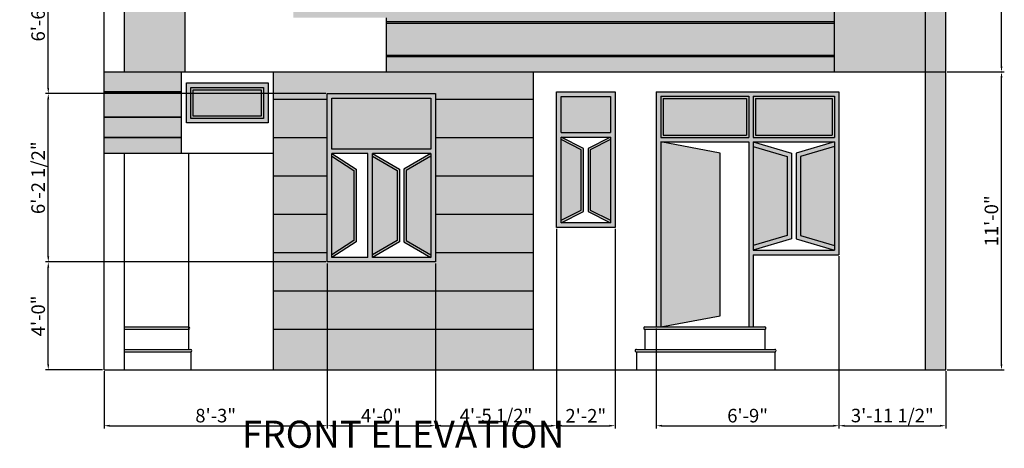
# Model space of a CAD drawing. Units: millimetres. Extents: x 4237 to 5109, y 21391 to 22486.
# Tile 1 of 17: x 4672 to 5109, y 21391 to 21581. Entities that reach past the tile are written whole.
import ezdxf

# ---------------------------------------------------------------- set-up
doc = ezdxf.new("R2010")
doc.units = ezdxf.units.MM
for name, color, linetype, lineweight in [('A-ANNO-DIMS', 2, 'Continuous', 18), ('A-ANNO-TEXT', 7, 'Continuous', 18), ('A-ELEV', 7, 'Continuous', 25), ('A-ELEV-PATT', 252, 'Continuous', 13)]:
    doc.layers.add(name, color=color, linetype=linetype, lineweight=lineweight)
doc.styles.get("Standard").update_dxf_attribs({"font": 'arial.ttf'})
doc.dimstyles.new('ISO-25', dxfattribs={"dimtxt": 6, "dimasz": 2.5, "dimexe": 1.25, "dimexo": 0.625, "dimtad": 1, "dimdec": 1, "dimlunit": 4, "dimtxsty": 'Standard', "dimcen": 2.5, "dimadec": 0, "dimazin": 0, "dimtfac": 1, "dimtdec": 1, "dimtmove": 0, "dimatfit": 3, "dimfxl": 1, "dimarcsym": 0})

# ---------------------------------------------------------------- blocks, each defined once
blk = doc.blocks.new('*D122')
at = {"layer": 'A-ANNO-DIMS', "color": 0, "lineweight": -2, "transparency": 16777216}
for p, q in [((4808.23, 21473.02), (4808.23, 21399.84)), ((4709.23, 21425.21), (4709.23, 21399.84)), ((4711.73, 21401.09), (4805.73, 21401.09))]:
    blk.add_line(p, q, dxfattribs=at)
at = {"layer": 'A-ANNO-DIMS', "color": 0, "transparency": 16777216}
for points in [[(4711.73, 21401.5), (4711.73, 21400.67), (4709.23, 21401.09)], [(4805.73, 21401.5), (4805.73, 21400.67), (4808.23, 21401.09)]]:
    blk.add_solid(points, dxfattribs=at)
at = {"layer": 'Defpoints', "color": 0, "transparency": 16777216}
for p in [(4808.23, 21473.65), (4709.23, 21425.84), (4808.23, 21401.09)]:
    blk.add_point(p, dxfattribs=at)
at = {"layer": 'A-ANNO-DIMS', "color": 0, "transparency": 16777216, "insert": (4758.73, 21404.78), "char_height": 6, "attachment_point": 5}
blk.add_mtext('8\'-3"', dxfattribs=at)
blk = doc.blocks.new('*D123')
at = {"layer": 'A-ANNO-DIMS', "color": 0, "lineweight": -2, "transparency": 16777216}
for p, q in [((4808.23, 21473.02), (4808.23, 21399.84)), ((4856.23, 21473.02), (4856.23, 21399.84)), ((4810.73, 21401.09), (4853.73, 21401.09))]:
    blk.add_line(p, q, dxfattribs=at)
at = {"layer": 'A-ANNO-DIMS', "color": 0, "transparency": 16777216}
for points in [[(4810.73, 21401.5), (4810.73, 21400.67), (4808.23, 21401.09)], [(4853.73, 21401.5), (4853.73, 21400.67), (4856.23, 21401.09)]]:
    blk.add_solid(points, dxfattribs=at)
at = {"layer": 'Defpoints', "color": 0, "transparency": 16777216}
for p in [(4808.23, 21473.65), (4856.23, 21473.65), (4856.23, 21401.09)]:
    blk.add_point(p, dxfattribs=at)
at = {"layer": 'A-ANNO-DIMS', "color": 0, "transparency": 16777216, "insert": (4832.23, 21404.77), "char_height": 6, "attachment_point": 5}
blk.add_mtext('4\'-0"', dxfattribs=at)
blk = doc.blocks.new('*D124')
at = {"layer": 'A-ANNO-DIMS', "color": 0, "lineweight": -2, "transparency": 16777216}
for p, q in [((4909.9, 21488.34), (4909.9, 21399.84)), ((4856.23, 21473.02), (4856.23, 21399.84)), ((4858.73, 21401.09), (4907.4, 21401.09))]:
    blk.add_line(p, q, dxfattribs=at)
at = {"layer": 'A-ANNO-DIMS', "color": 0, "transparency": 16777216}
for points in [[(4858.73, 21401.5), (4858.73, 21400.67), (4856.23, 21401.09)], [(4907.4, 21401.5), (4907.4, 21400.67), (4909.9, 21401.09)]]:
    blk.add_solid(points, dxfattribs=at)
at = {"layer": 'Defpoints', "color": 0, "transparency": 16777216}
for p in [(4909.9, 21488.97), (4856.23, 21473.65), (4909.9, 21401.09)]:
    blk.add_point(p, dxfattribs=at)
at = {"layer": 'A-ANNO-DIMS', "color": 0, "transparency": 16777216, "insert": (4883.06, 21404.81), "char_height": 6, "attachment_point": 5}
blk.add_mtext('4\'-5 1/2"', dxfattribs=at)
blk = doc.blocks.new('*D125')
at = {"layer": 'A-ANNO-DIMS', "color": 0, "lineweight": -2, "transparency": 16777216}
for p, q in [((4909.9, 21488.34), (4909.9, 21399.84)), ((4935.9, 21488.34), (4935.9, 21399.84)), ((4912.4, 21401.09), (4933.4, 21401.09))]:
    blk.add_line(p, q, dxfattribs=at)
at = {"layer": 'A-ANNO-DIMS', "color": 0, "transparency": 16777216}
for points in [[(4912.4, 21401.5), (4912.4, 21400.67), (4909.9, 21401.09)], [(4933.4, 21401.5), (4933.4, 21400.67), (4935.9, 21401.09)]]:
    blk.add_solid(points, dxfattribs=at)
at = {"layer": 'Defpoints', "color": 0, "transparency": 16777216}
for p in [(4909.9, 21488.97), (4935.9, 21488.97), (4935.9, 21401.09)]:
    blk.add_point(p, dxfattribs=at)
at = {"layer": 'A-ANNO-DIMS', "color": 0, "transparency": 16777216, "insert": (4922.9, 21404.72), "char_height": 6, "attachment_point": 5}
blk.add_mtext('2\'-2"', dxfattribs=at)
blk = doc.blocks.new('*D126')
at = {"layer": 'A-ANNO-DIMS', "color": 0, "lineweight": -2, "transparency": 16777216}
for p, q in [((5035.17, 21476.21), (5035.17, 21399.84)), ((4954.17, 21444.21), (4954.17, 21399.84)), ((4956.67, 21401.09), (5032.67, 21401.09))]:
    blk.add_line(p, q, dxfattribs=at)
at = {"layer": 'A-ANNO-DIMS', "color": 0, "transparency": 16777216}
for points in [[(4956.67, 21401.5), (4956.67, 21400.67), (4954.17, 21401.09)], [(5032.67, 21401.5), (5032.67, 21400.67), (5035.17, 21401.09)]]:
    blk.add_solid(points, dxfattribs=at)
at = {"layer": 'Defpoints', "color": 0, "transparency": 16777216}
for p in [(5035.17, 21476.84), (4954.17, 21444.84), (5035.17, 21401.09)]:
    blk.add_point(p, dxfattribs=at)
at = {"layer": 'A-ANNO-DIMS', "color": 0, "transparency": 16777216, "insert": (4994.67, 21404.77), "char_height": 6, "attachment_point": 5}
blk.add_mtext('6\'-9"', dxfattribs=at)
blk = doc.blocks.new('*D127')
at = {"layer": 'A-ANNO-DIMS', "color": 0, "lineweight": -2, "transparency": 16777216}
for p, q in [((5035.17, 21476.21), (5035.17, 21399.84)), ((5082.53, 21425.21), (5082.53, 21399.84)), ((5037.67, 21401.09), (5080.03, 21401.09))]:
    blk.add_line(p, q, dxfattribs=at)
at = {"layer": 'A-ANNO-DIMS', "color": 0, "transparency": 16777216}
for points in [[(5037.67, 21401.5), (5037.67, 21400.67), (5035.17, 21401.09)], [(5080.03, 21401.5), (5080.03, 21400.67), (5082.53, 21401.09)]]:
    blk.add_solid(points, dxfattribs=at)
at = {"layer": 'Defpoints', "color": 0, "transparency": 16777216}
for p in [(5035.17, 21476.84), (5082.53, 21425.84), (5082.53, 21401.09)]:
    blk.add_point(p, dxfattribs=at)
at = {"layer": 'A-ANNO-DIMS', "color": 0, "transparency": 16777216, "insert": (5058.85, 21404.82), "char_height": 6, "attachment_point": 5}
blk.add_mtext('3\'-11 1/2"', dxfattribs=at)
blk = doc.blocks.new('*D128')
at = {"layer": 'A-ANNO-DIMS', "color": 0, "lineweight": -2, "transparency": 16777216}
for p, q in [((4709.23, 21558.46), (4709.23, 21897.84)), ((4800.45, 21688.54), (4800.45, 21897.84)), ((4711.73, 21896.59), (4797.95, 21896.59))]:
    blk.add_line(p, q, dxfattribs=at)
at = {"layer": 'A-ANNO-DIMS', "color": 0, "transparency": 16777216}
for points in [[(4711.73, 21897), (4711.73, 21896.17), (4709.23, 21896.59)], [(4797.95, 21897), (4797.95, 21896.17), (4800.45, 21896.59)]]:
    blk.add_solid(points, dxfattribs=at)
at = {"layer": 'Defpoints', "color": 0, "transparency": 16777216}
for p in [(4800.45, 21896.59), (4800.45, 21687.91), (4709.23, 21557.84)]:
    blk.add_point(p, dxfattribs=at)
at = {"layer": 'A-ANNO-DIMS', "color": 0, "transparency": 16777216, "insert": (4754.84, 21900.21), "char_height": 6, "attachment_point": 5}
blk.add_mtext('7\'-7"', dxfattribs=at)
blk = doc.blocks.new('*D135')
at = {"layer": 'A-ANNO-DIMS', "color": 0, "lineweight": -2, "transparency": 16777216}
for p, q in [((5083.15, 21557.84), (5108.53, 21557.84)), ((5107.28, 21428.34), (5107.28, 21555.34)), ((5083.15, 21425.84), (5108.53, 21425.84))]:
    blk.add_line(p, q, dxfattribs=at)
at = {"layer": 'A-ANNO-DIMS', "color": 0, "transparency": 16777216}
for points in [[(5106.86, 21555.34), (5107.69, 21555.34), (5107.28, 21557.84)], [(5106.86, 21428.34), (5107.69, 21428.34), (5107.28, 21425.84)]]:
    blk.add_solid(points, dxfattribs=at)
at = {"layer": 'Defpoints', "color": 0, "transparency": 16777216}
for p in [(5082.53, 21557.84), (5107.28, 21557.84), (5082.53, 21425.84)]:
    blk.add_point(p, dxfattribs=at)
at = {"layer": 'A-ANNO-DIMS', "color": 0, "transparency": 16777216, "insert": (5103.59, 21491.84), "char_height": 6, "attachment_point": 5, "rotation": 90}
blk.add_mtext('11\'-0"', dxfattribs=at)
blk = doc.blocks.new('*D136')
at = {"layer": 'A-ANNO-DIMS', "color": 0, "lineweight": -2, "transparency": 16777216}
for p, q in [((5074.15, 21727.84), (5108.53, 21727.84)), ((5107.28, 21560.34), (5107.28, 21725.34)), ((5083.15, 21557.84), (5108.53, 21557.84))]:
    blk.add_line(p, q, dxfattribs=at)
at = {"layer": 'A-ANNO-DIMS', "color": 0, "transparency": 16777216}
for points in [[(5106.86, 21725.34), (5107.69, 21725.34), (5107.28, 21727.84)], [(5106.86, 21560.34), (5107.69, 21560.34), (5107.28, 21557.84)]]:
    blk.add_solid(points, dxfattribs=at)
at = {"layer": 'Defpoints', "color": 0, "transparency": 16777216}
for p in [(5073.53, 21727.84), (5107.28, 21727.84), (5082.53, 21557.84)]:
    blk.add_point(p, dxfattribs=at)
at = {"layer": 'A-ANNO-DIMS', "color": 0, "transparency": 16777216, "insert": (5103.64, 21642.84), "char_height": 6, "attachment_point": 5, "rotation": 90}
blk.add_mtext('14\'-2"', dxfattribs=at)
blk = doc.blocks.new('*D138')
at = {"layer": 'A-ANNO-DIMS', "color": 0, "lineweight": -2, "transparency": 16777216}
for p, q in [((4807.6, 21473.65), (4683.23, 21473.65)), ((4684.48, 21428.34), (4684.48, 21471.15)), ((4708.6, 21425.84), (4683.23, 21425.84))]:
    blk.add_line(p, q, dxfattribs=at)
at = {"layer": 'A-ANNO-DIMS', "color": 0, "transparency": 16777216}
for points in [[(4684.06, 21471.15), (4684.89, 21471.15), (4684.48, 21473.65)], [(4684.06, 21428.34), (4684.89, 21428.34), (4684.48, 21425.84)]]:
    blk.add_solid(points, dxfattribs=at)
at = {"layer": 'Defpoints', "color": 0, "transparency": 16777216}
for p in [(4684.48, 21473.65), (4808.23, 21473.65), (4709.23, 21425.84)]:
    blk.add_point(p, dxfattribs=at)
at = {"layer": 'A-ANNO-DIMS', "color": 0, "transparency": 16777216, "insert": (4680.79, 21449.74), "char_height": 6, "attachment_point": 5, "rotation": 90}
blk.add_mtext('4\'-0"', dxfattribs=at)
blk = doc.blocks.new('*D139')
at = {"layer": 'A-ANNO-DIMS', "color": 0, "lineweight": -2, "transparency": 16777216}
for p, q in [((4807.6, 21548.26), (4683.23, 21548.26)), ((4684.48, 21476.15), (4684.48, 21545.76)), ((4807.6, 21473.65), (4683.23, 21473.65))]:
    blk.add_line(p, q, dxfattribs=at)
at = {"layer": 'A-ANNO-DIMS', "color": 0, "transparency": 16777216}
for points in [[(4684.06, 21545.76), (4684.89, 21545.76), (4684.48, 21548.26)], [(4684.06, 21476.15), (4684.89, 21476.15), (4684.48, 21473.65)]]:
    blk.add_solid(points, dxfattribs=at)
at = {"layer": 'Defpoints', "color": 0, "transparency": 16777216}
for p in [(4684.48, 21548.26), (4808.23, 21548.26), (4808.23, 21473.65)]:
    blk.add_point(p, dxfattribs=at)
at = {"layer": 'A-ANNO-DIMS', "color": 0, "transparency": 16777216, "insert": (4680.75, 21510.96), "char_height": 6, "attachment_point": 5, "rotation": 90}
blk.add_mtext('6\'-2 1/2"', dxfattribs=at)
blk = doc.blocks.new('*D140')
at = {"layer": 'A-ANNO-DIMS', "color": 0, "lineweight": -2, "transparency": 16777216}
for p, q in [((4799.82, 21626.61), (4683.23, 21626.61)), ((4684.48, 21550.76), (4684.48, 21624.11)), ((4807.6, 21548.26), (4683.23, 21548.26))]:
    blk.add_line(p, q, dxfattribs=at)
at = {"layer": 'A-ANNO-DIMS', "color": 0, "transparency": 16777216}
for points in [[(4684.06, 21624.11), (4684.89, 21624.11), (4684.48, 21626.61)], [(4684.06, 21550.76), (4684.89, 21550.76), (4684.48, 21548.26)]]:
    blk.add_solid(points, dxfattribs=at)
at = {"layer": 'Defpoints', "color": 0, "transparency": 16777216}
for p in [(4684.48, 21626.61), (4800.45, 21626.61), (4808.23, 21548.26)]:
    blk.add_point(p, dxfattribs=at)
at = {"layer": 'A-ANNO-DIMS', "color": 0, "transparency": 16777216, "insert": (4680.75, 21587.44), "char_height": 6, "attachment_point": 5, "rotation": 90}
blk.add_mtext('6\'-6 1/2"', dxfattribs=at)

msp = doc.modelspace()

# ---------------------------------------------------------------- hatches: boundary and pattern name
at = {"layer": 'A-ELEV-PATT'}
h = msp.add_hatch(color=256, dxfattribs=at)
h.dxf.hatch_style = 1
h.paths.add_polyline_path([(4957.45, 21796.84), (4963.45, 21796.84), (4963.45, 21727.84), (4966.45, 21727.84), (4966.45, 21796.84), (4972.45, 21796.84), (4972.45, 21727.84), (4975.45, 21727.84), (4975.45, 21796.84), (4981.45, 21796.84), (4981.45, 21727.84), (4984.45, 21727.84), (4984.45, 21796.84), (5073.53, 21796.84), (5073.53, 21557.84), (5082.53, 21557.84), (5082.53, 21808.84), (4951.45, 21808.84), (4951.45, 21727.84), (4957.45, 21727.84)])
h = msp.add_hatch(color=256, dxfattribs=at)
h.dxf.hatch_style = 1
h.paths.add_polyline_path([(4763.12, 21763.84), (4718.23, 21763.84), (4718.23, 21557.84), (4745.15, 21557.84), (4745.15, 21725.84), (4742.84, 21725.84), (4742.84, 21727.84), (4763.12, 21727.84)])
h = msp.add_hatch(color=256, dxfattribs=at)
h.dxf.hatch_style = 1
h.paths.add_polyline_path([(5073.53, 21725.84), (5033.17, 21725.84), (5033.17, 21557.84), (5073.53, 21557.84)])
h = msp.add_hatch(color=256, dxfattribs=at)
h.dxf.hatch_style = 1
h.paths.add_polyline_path([(5033.17, 21587.38), (4793.12, 21587.38), (4793.12, 21581.84), (4834.56, 21581.84), (4834.56, 21580.12), (5033.17, 21580.12)])
h = msp.add_hatch(color=256, dxfattribs=at)
h.dxf.hatch_style = 1
h.paths.add_polyline_path([(5033.17, 21580.12), (4834.56, 21580.12), (4834.56, 21579.49), (5033.17, 21579.49)])
h = msp.add_hatch(color=256, dxfattribs=at)
h.dxf.hatch_style = 1
h.paths.add_polyline_path([(5033.17, 21579.49), (4834.56, 21579.49), (4834.56, 21565.26), (5033.17, 21565.26)])
h = msp.add_hatch(color=256, dxfattribs=at)
h.dxf.hatch_style = 1
h.paths.add_polyline_path([(5033.17, 21565.26), (4834.56, 21565.26), (4834.56, 21564.63), (5033.17, 21564.63)])
h = msp.add_hatch(color=256, dxfattribs=at)
h.dxf.hatch_style = 1
h.paths.add_polyline_path([(5033.17, 21564.63), (4834.56, 21564.63), (4834.56, 21557.84), (5033.17, 21557.84)])
h = msp.add_hatch(color=256, dxfattribs=at)
h.dxf.hatch_style = 1
h.paths.add_polyline_path([(4743.58, 21557.84), (4709.23, 21557.84), (4709.23, 21521.84), (4743.58, 21521.84)])
h = msp.add_hatch(color=256, dxfattribs=at)
h.dxf.hatch_style = 1
h.paths.add_polyline_path([(4899.53, 21557.84), (4784.23, 21557.84), (4784.23, 21425.84), (4899.53, 21425.84)])
h.paths.add_polyline_path([(4808.23, 21473.65), (4808.23, 21548.26), (4856.23, 21548.26), (4856.23, 21473.65)], flags=16)
h.paths.add_polyline_path([(4810.23, 21475.65), (4810.23, 21521.65), (4826.23, 21521.65), (4826.23, 21475.65)], flags=0)
h.paths.add_polyline_path([(4828.23, 21475.65), (4828.23, 21521.65), (4854.23, 21521.65), (4854.23, 21475.65)], flags=0)
h.paths.add_polyline_path([(4810.23, 21523.65), (4810.23, 21546.26), (4854.23, 21546.26), (4854.23, 21523.65)], flags=0)
h = msp.add_hatch(color=256, dxfattribs=at)
h.dxf.hatch_style = 1
h.paths.add_polyline_path([(5082.53, 21557.84), (5073.53, 21557.84), (5073.53, 21425.84), (5082.53, 21425.84)])
h = msp.add_hatch(color=256, dxfattribs=at)
h.dxf.hatch_style = 1
h.paths.add_polyline_path([(4781.97, 21552.96), (4745.76, 21552.96), (4745.76, 21535.28), (4781.97, 21535.28)])
h.paths.add_polyline_path([(4747.76, 21537.28), (4747.76, 21550.96), (4779.97, 21550.96), (4779.97, 21537.28)], flags=16)
h.paths.add_polyline_path([(4748.76, 21538.28), (4748.76, 21549.96), (4778.97, 21549.96), (4778.97, 21538.28)], flags=0)
h = msp.add_hatch(color=256, dxfattribs=at)
h.dxf.hatch_style = 1
h.set_gradient(color1=(122, 175, 223), color2=(215, 235, 210), name='CYLINDER')
h.paths.add_polyline_path([(4779.97, 21550.96), (4747.76, 21550.96), (4747.76, 21537.28), (4779.97, 21537.28)])
h.paths.add_polyline_path([(4778.97, 21538.28), (4748.76, 21538.28), (4748.76, 21549.96), (4778.97, 21549.96)], flags=16)
h = msp.add_hatch(color=256, dxfattribs=at)
h.dxf.hatch_style = 1
h.set_gradient(color1=(122, 175, 223), color2=(215, 235, 210), name='HEMISPHERICAL')
h.paths.add_polyline_path([(4778.97, 21549.96), (4748.76, 21549.96), (4748.76, 21538.28), (4778.97, 21538.28)])
h = msp.add_hatch(color=256, dxfattribs=at)
h.dxf.hatch_style = 1
h.paths.add_polyline_path([(4856.23, 21548.26), (4808.23, 21548.26), (4808.23, 21473.65), (4856.23, 21473.65)])
h.paths.add_polyline_path([(4854.23, 21546.26), (4854.23, 21523.65), (4810.23, 21523.65), (4810.23, 21546.26)], flags=16)
h.paths.add_polyline_path([(4854.23, 21521.65), (4854.23, 21475.65), (4828.23, 21475.65), (4828.23, 21521.65)], flags=16)
h.paths.add_polyline_path([(4826.23, 21521.65), (4826.23, 21475.65), (4810.23, 21475.65), (4810.23, 21521.65)], flags=16)
h = msp.add_hatch(color=256, dxfattribs=at)
h.dxf.hatch_style = 1
h.paths.add_polyline_path([(4935.9, 21548.97), (4909.9, 21548.97), (4909.9, 21488.97), (4935.9, 21488.97)])
h.paths.add_polyline_path([(4933.9, 21546.97), (4933.9, 21530.97), (4911.9, 21530.97), (4911.9, 21546.97)], flags=16)
h.paths.add_polyline_path([(4933.9, 21528.97), (4933.9, 21490.97), (4911.9, 21490.97), (4911.9, 21528.97)], flags=16)
h = msp.add_hatch(color=256, dxfattribs=at)
h.dxf.hatch_style = 1
h.paths.add_polyline_path([(5035.17, 21549.03), (4954.17, 21549.03), (4954.17, 21444.84), (4956.17, 21444.84), (4956.17, 21526.84), (4995.17, 21526.84), (4995.17, 21444.84), (4997.17, 21444.84), (4997.17, 21476.84), (5035.17, 21476.84)])
h.paths.add_polyline_path([(4995.17, 21547.03), (4995.17, 21528.84), (4956.17, 21528.84), (4956.17, 21547.03)], flags=16)
h.paths.add_polyline_path([(4994.17, 21546.03), (4994.17, 21529.84), (4957.17, 21529.84), (4957.17, 21546.03)], flags=0)
h.paths.add_polyline_path([(4997.17, 21547.03), (5033.17, 21547.03), (5033.17, 21528.84), (4997.17, 21528.84)], flags=16)
h.paths.add_polyline_path([(4998.17, 21546.03), (5032.17, 21546.03), (5032.17, 21529.84), (4998.17, 21529.84)], flags=0)
h.paths.add_polyline_path([(4997.17, 21526.84), (5033.17, 21526.84), (5033.17, 21478.84), (4997.17, 21478.84)], flags=16)
h = msp.add_hatch(color=256, dxfattribs=at)
h.dxf.hatch_style = 1
h.set_gradient(color1=(122, 175, 223), color2=(215, 235, 210), name='HEMISPHERICAL')
h.paths.add_polyline_path([(4854.23, 21546.26), (4810.23, 21546.26), (4810.23, 21523.65), (4854.23, 21523.65)])
h = msp.add_hatch(color=256, dxfattribs=at)
h.dxf.hatch_style = 1
h.set_gradient(color1=(122, 175, 223), color2=(215, 235, 210), name='HEMISPHERICAL')
h.paths.add_polyline_path([(4933.9, 21546.97), (4911.9, 21546.97), (4911.9, 21530.97), (4933.9, 21530.97)])
h = msp.add_hatch(color=256, dxfattribs=at)
h.dxf.hatch_style = 1
h.set_gradient(color1=(122, 175, 223), color2=(215, 235, 210), name='CYLINDER')
h.paths.add_polyline_path([(4995.17, 21547.03), (4956.17, 21547.03), (4956.17, 21528.84), (4995.17, 21528.84)])
h.paths.add_polyline_path([(4994.17, 21529.84), (4957.17, 21529.84), (4957.17, 21546.03), (4994.17, 21546.03)], flags=16)
h = msp.add_hatch(color=256, dxfattribs=at)
h.dxf.hatch_style = 1
h.set_gradient(color1=(122, 175, 223), color2=(215, 235, 210), name='HEMISPHERICAL')
h.paths.add_polyline_path([(4994.17, 21546.03), (4957.17, 21546.03), (4957.17, 21529.84), (4994.17, 21529.84)])
h = msp.add_hatch(color=256, dxfattribs=at)
h.dxf.hatch_style = 1
h.set_gradient(color1=(122, 175, 223), color2=(215, 235, 210), name='CYLINDER')
h.paths.add_polyline_path([(5033.17, 21547.03), (4997.17, 21547.03), (4997.17, 21528.84), (5033.17, 21528.84)])
h.paths.add_polyline_path([(4998.17, 21546.03), (5032.17, 21546.03), (5032.17, 21529.84), (4998.17, 21529.84)], flags=16)
h = msp.add_hatch(color=256, dxfattribs=at)
h.dxf.hatch_style = 1
h.set_gradient(color1=(122, 175, 223), color2=(215, 235, 210), name='HEMISPHERICAL')
h.paths.add_polyline_path([(5032.17, 21546.03), (4998.17, 21546.03), (4998.17, 21529.84), (5032.17, 21529.84)])
h = msp.add_hatch(color=256, dxfattribs=at)
h.dxf.hatch_style = 1
h.paths.add_polyline_path([(4921.9, 21523.97), (4911.9, 21528.97), (4911.9, 21527.85), (4920.9, 21523.35), (4920.9, 21496.59), (4911.9, 21492.09), (4911.9, 21490.97), (4921.9, 21495.97)])
h = msp.add_hatch(color=256, dxfattribs=at)
h.dxf.hatch_style = 1
h.set_gradient(color1=(122, 175, 223), color2=(215, 235, 210), name='INVCYLINDER')
h.paths.add_polyline_path([(4920.9, 21523.35), (4911.9, 21527.85), (4911.9, 21492.09), (4920.9, 21496.59)])
h = msp.add_hatch(color=256, dxfattribs=at)
h.dxf.hatch_style = 1
h.paths.add_polyline_path([(4924.9, 21523.35), (4933.9, 21527.85), (4933.9, 21528.97), (4923.9, 21523.97), (4923.9, 21495.97), (4933.9, 21490.97), (4933.9, 21492.09), (4924.9, 21496.59)])
h = msp.add_hatch(color=256, dxfattribs=at)
h.dxf.hatch_style = 1
h.set_gradient(color1=(122, 175, 223), color2=(215, 235, 210), name='INVCYLINDER')
h.paths.add_polyline_path([(4933.9, 21527.85), (4924.9, 21523.35), (4924.9, 21496.59), (4933.9, 21492.09)])
h = msp.add_hatch(color=256, dxfattribs=at)
h.dxf.hatch_style = 1
h.paths.add_polyline_path([(4982.51, 21521.84), (4956.17, 21526.84), (4956.17, 21444.84), (4982.51, 21449.84)])
h = msp.add_hatch(color=256, dxfattribs=at)
h.dxf.hatch_style = 1
h.paths.add_polyline_path([(5014.17, 21521.84), (4997.17, 21526.84), (4997.17, 21524.75), (5012.17, 21520.34), (5012.17, 21485.33), (4997.17, 21480.92), (4997.17, 21478.84), (5014.17, 21483.84)])
h = msp.add_hatch(color=256, dxfattribs=at)
h.dxf.hatch_style = 1
h.paths.add_polyline_path([(5018.17, 21520.34), (5033.17, 21524.75), (5033.17, 21526.84), (5016.17, 21521.84), (5016.17, 21483.84), (5033.17, 21478.84), (5033.17, 21480.92), (5018.17, 21485.33)])
h = msp.add_hatch(color=256, dxfattribs=at)
h.dxf.hatch_style = 1
h.set_gradient(color1=(122, 175, 223), color2=(215, 235, 210), name='INVCYLINDER')
h.paths.add_polyline_path([(5012.17, 21520.34), (4997.17, 21524.75), (4997.17, 21480.92), (5012.17, 21485.33)])
h = msp.add_hatch(color=256, dxfattribs=at)
h.dxf.hatch_style = 1
h.set_gradient(color1=(122, 175, 223), color2=(215, 235, 210), name='INVCYLINDER')
h.paths.add_polyline_path([(5033.17, 21524.75), (5018.17, 21520.34), (5018.17, 21485.33), (5033.17, 21480.92)])
h = msp.add_hatch(color=256, dxfattribs=at)
h.dxf.hatch_style = 1
h.paths.add_polyline_path([(4821, 21514.73), (4810.23, 21521.65), (4810.23, 21520.46), (4820, 21514.19), (4820, 21483.11), (4810.23, 21476.84), (4810.23, 21475.65), (4821, 21482.56)])
h = msp.add_hatch(color=256, dxfattribs=at)
h.dxf.hatch_style = 1
h.set_gradient(color1=(122, 175, 223), color2=(215, 235, 210), name='INVCYLINDER')
h.paths.add_polyline_path([(4820, 21514.19), (4810.23, 21520.46), (4810.23, 21476.84), (4820, 21483.11)])
h = msp.add_hatch(color=256, dxfattribs=at)
h.dxf.hatch_style = 1
h.paths.add_polyline_path([(4840.21, 21514.73), (4828.23, 21521.65), (4828.23, 21520.49), (4839.21, 21514.16), (4839.21, 21483.14), (4828.23, 21476.8), (4828.23, 21475.65), (4840.21, 21482.56)])
h = msp.add_hatch(color=256, dxfattribs=at)
h.dxf.hatch_style = 1
h.set_gradient(color1=(122, 175, 223), color2=(215, 235, 210), name='INVCYLINDER')
h.paths.add_polyline_path([(4839.21, 21514.16), (4828.23, 21520.49), (4828.23, 21476.8), (4839.21, 21483.14)])
h = msp.add_hatch(color=256, dxfattribs=at)
h.dxf.hatch_style = 1
h.paths.add_polyline_path([(4843.24, 21514.16), (4854.23, 21520.49), (4854.23, 21521.65), (4842.24, 21514.73), (4842.24, 21482.56), (4854.23, 21475.65), (4854.23, 21476.8), (4843.24, 21483.14)])
h = msp.add_hatch(color=256, dxfattribs=at)
h.dxf.hatch_style = 1
h.set_gradient(color1=(122, 175, 223), color2=(215, 235, 210), name='INVCYLINDER')
h.paths.add_polyline_path([(4854.23, 21520.49), (4843.24, 21514.16), (4843.24, 21483.14), (4854.23, 21476.8)])

# ---------------------------------------------------------------- linework, layer by layer
at = {"layer": 'A-ELEV'}
for p, q in [((4709.23, 21425.84), (4709.23, 21871.84)), ((5082.53, 21425.84), (5082.53, 21808.84)), ((5073.53, 21425.84), (5073.53, 21796.84)), ((5033.17, 21557.84), (5033.17, 21772.84)), ((4718.23, 21557.84), (4718.23, 21763.84)), ((4745.15, 21557.84), (4745.15, 21725.84)), ((4834.56, 21557.84), (4834.56, 21581.84)), ((4834.56, 21580.12), (5033.17, 21580.12)), ((4834.56, 21579.49), (5033.17, 21579.49)), ((4834.56, 21565.26), (5033.17, 21565.26)), ((4834.56, 21564.63), (5033.17, 21564.63)), ((4709.23, 21557.84), (5082.53, 21557.84)), ((4743.58, 21521.84), (4743.58, 21557.84)), ((4784.23, 21557.84), (4784.23, 21425.84)), ((4899.53, 21557.84), (4899.53, 21425.84)), ((4709.23, 21549.12), (4743.58, 21549.12)), ((4709.23, 21548.93), (4743.58, 21548.93)), ((4808.23, 21548.26), (4856.23, 21548.26)), ((4808.23, 21473.65), (4808.23, 21548.26)), ((4856.23, 21548.26), (4856.23, 21473.65)), ((4909.9, 21548.97), (4935.9, 21548.97)), ((4909.9, 21488.97), (4909.9, 21548.97)), ((4935.9, 21548.97), (4935.9, 21488.97)), ((4954.17, 21549.03), (4954.17, 21444.84)), ((4954.17, 21549.03), (5035.17, 21549.03)), ((5035.17, 21549.03), (5035.17, 21476.84)), ((4784.23, 21545.84), (4808.23, 21545.84)), ((4856.23, 21545.84), (4899.53, 21545.84)), ((4911.9, 21546.97), (4933.9, 21546.97)), ((4911.9, 21530.97), (4911.9, 21546.97)), ((4933.9, 21546.97), (4933.9, 21530.97)), ((4956.17, 21547.03), (4956.17, 21528.84)), ((4956.17, 21547.03), (4995.17, 21547.03)), ((4957.17, 21546.03), (4957.17, 21529.84)), ((4957.17, 21546.03), (4994.17, 21546.03)), ((4994.17, 21546.03), (4994.17, 21529.84)), ((4995.17, 21547.03), (4995.17, 21528.84)), ((4997.17, 21547.03), (4997.17, 21528.84)), ((4997.17, 21547.03), (5033.17, 21547.03)), ((4998.17, 21546.03), (4998.17, 21529.84)), ((4998.17, 21546.03), (5032.17, 21546.03)), ((5032.17, 21546.03), (5032.17, 21529.84)), ((5033.17, 21547.03), (5033.17, 21528.84)), ((4709.23, 21537.93), (4743.58, 21537.93)), ((4709.23, 21537.73), (4743.58, 21537.73)), ((4911.9, 21530.97), (4933.9, 21530.97)), ((4709.23, 21529.01), (4743.58, 21529.01)), ((4709.23, 21528.81), (4743.58, 21528.81)), ((4784.23, 21528.84), (4808.23, 21528.84)), ((4856.23, 21528.84), (4899.53, 21528.84)), ((4911.9, 21528.97), (4933.9, 21528.97)), ((4911.9, 21490.97), (4911.9, 21528.97)), ((4933.9, 21528.97), (4933.9, 21490.97)), ((4956.17, 21528.84), (4995.17, 21528.84)), ((4956.17, 21526.84), (4995.17, 21526.84)), ((4956.17, 21526.84), (4956.17, 21444.84)), ((4957.17, 21529.84), (4994.17, 21529.84)), ((4995.17, 21526.84), (4995.17, 21444.84)), ((4997.17, 21528.84), (5033.17, 21528.84)), ((4997.17, 21526.84), (5033.17, 21526.84)), ((4997.17, 21526.84), (4997.17, 21478.84)), ((4998.17, 21529.84), (5032.17, 21529.84)), ((5033.17, 21526.84), (5033.17, 21478.84)), ((4709.23, 21521.84), (4784.23, 21521.84)), ((4718.23, 21425.84), (4718.23, 21521.84)), ((4746.73, 21521.84), (4746.73, 21434.84)), ((4826.23, 21521.65), (4810.23, 21521.65)), ((4810.23, 21475.65), (4810.23, 21521.65)), ((4826.23, 21475.65), (4826.23, 21521.65)), ((4854.23, 21521.65), (4828.23, 21521.65)), ((4828.23, 21475.65), (4828.23, 21521.65)), ((4854.23, 21521.65), (4854.23, 21475.65)), ((4784.23, 21511.84), (4808.23, 21511.84)), ((4856.23, 21511.84), (4899.53, 21511.84)), ((4784.23, 21494.84), (4808.23, 21494.84)), ((4856.23, 21494.84), (4899.53, 21494.84)), ((4935.9, 21488.97), (4909.9, 21488.97)), ((4933.9, 21490.97), (4911.9, 21490.97)), ((4997.17, 21478.84), (5033.17, 21478.84)), ((4784.23, 21477.84), (4808.23, 21477.84)), ((4826.23, 21475.65), (4810.23, 21475.65)), ((4854.23, 21475.65), (4828.23, 21475.65)), ((4856.23, 21477.84), (4899.53, 21477.84)), ((4997.17, 21476.84), (5035.17, 21476.84)), ((4997.17, 21476.84), (4997.17, 21444.84)), ((4856.23, 21473.65), (4808.23, 21473.65)), ((4784.23, 21460.84), (4899.53, 21460.84)), ((4718.23, 21444.84), (4746.73, 21444.84)), ((4718.23, 21443.84), (4746.73, 21443.84)), ((4784.23, 21443.84), (4899.53, 21443.84)), ((4949.12, 21444.84), (5002.27, 21444.84)), ((4949.12, 21443.84), (5002.27, 21443.84)), ((4949.12, 21443.84), (4949.12, 21434.84)), ((5002.27, 21443.84), (5002.27, 21434.84)), ((4718.23, 21434.84), (4747.69, 21434.84)), ((4945.37, 21434.84), (5006.68, 21434.84)), ((4718.23, 21433.84), (4747.69, 21433.84)), ((4747.69, 21433.84), (4747.69, 21425.84)), ((4945.37, 21433.84), (5006.68, 21433.84)), ((4945.37, 21433.84), (4945.37, 21425.84)), ((5006.68, 21433.84), (5006.68, 21425.84)), ((4709.23, 21425.84), (5082.53, 21425.84))]:
    msp.add_line(p, q, dxfattribs=at)
for points in [[(4745.76, 21552.96), (4781.97, 21552.96), (4781.97, 21535.28), (4745.76, 21535.28)], [(4747.76, 21550.96), (4779.97, 21550.96), (4779.97, 21537.28), (4747.76, 21537.28)], [(4748.76, 21549.96), (4778.97, 21549.96), (4778.97, 21538.28), (4748.76, 21538.28)], [(4810.23, 21546.26), (4854.23, 21546.26), (4854.23, 21523.65), (4810.23, 21523.65)]]:
    msp.add_lwpolyline(points, close=True, dxfattribs=at)
for points in [[(4911.9, 21490.97), (4921.9, 21495.97), (4921.9, 21523.97), (4911.9, 21528.97)], [(4911.9, 21492.09), (4920.9, 21496.59), (4920.9, 21523.35), (4911.9, 21527.85)], [(4933.9, 21528.97), (4923.9, 21523.97), (4923.9, 21495.97), (4933.9, 21490.97)], [(4933.9, 21527.85), (4924.9, 21523.35), (4924.9, 21496.59), (4933.9, 21492.09)], [(4956.17, 21444.84), (4982.51, 21449.84), (4982.51, 21521.84), (4956.17, 21526.84)], [(4997.17, 21526.84), (5014.17, 21521.84), (5014.17, 21483.84), (4997.17, 21478.84)], [(5033.17, 21526.84), (5016.17, 21521.84), (5016.17, 21483.84), (5033.17, 21478.84)], [(4997.17, 21524.75), (5012.17, 21520.34), (5012.17, 21485.33), (4997.17, 21480.92)], [(5033.17, 21524.75), (5018.17, 21520.34), (5018.17, 21485.33), (5033.17, 21480.92)], [(4810.23, 21521.65), (4821, 21514.73), (4821, 21482.56), (4810.23, 21475.65)], [(4810.23, 21520.46), (4820, 21514.19), (4820, 21483.11), (4810.23, 21476.84)], [(4828.23, 21521.65), (4840.21, 21514.73), (4840.21, 21482.56), (4828.23, 21475.65)], [(4828.23, 21520.49), (4839.21, 21514.16), (4839.21, 21483.14), (4828.23, 21476.8)], [(4854.23, 21521.65), (4842.24, 21514.73), (4842.24, 21482.56), (4854.23, 21475.65)], [(4854.23, 21520.49), (4843.24, 21514.16), (4843.24, 21483.14), (4854.23, 21476.8)]]:
    msp.add_lwpolyline(points, dxfattribs=at)
for centre, radius, start, end in [((4746.74, 21444.34), 0.5, 268.0101, 91.9899), ((4949.08, 21444.34), 0.502, 84.9128, 275.0872), ((5002.31, 21444.34), 0.502, 264.751, 95.249), ((4747.69, 21434.34), 0.5, 270.7076, 89.2924), ((4945.24, 21434.34), 0.517, 75.0765, 284.9235), ((5006.77, 21434.34), 0.51, 258.8891, 101.1109)]:
    msp.add_arc(centre, radius, start, end, dxfattribs=at)

# ---------------------------------------------------------------- texts
at = {"layer": 'A-ANNO-TEXT', "insert": (4755.67, 21403.3), "char_height": 12, "attachment_point": 1}
msp.add_mtext_dynamic_manual_height_columns('    FRONT ELEVATION', width=222.3103, gutter_width=12.5, heights=[0], dxfattribs=at)

# ---------------------------------------------------------------- dimensions: what is measured, and where the dimension line sits
at = {"layer": 'A-ANNO-DIMS'}
for base, p1, p2, picture, middle in [((4800.45, 21896.59), (4709.23, 21557.84), (4800.45, 21687.91), '*D128', (4754.84, 21900.21)), ((4909.9, 21401.09), (4856.23, 21473.65), (4909.9, 21488.97), '*D124', (4883.06, 21404.81)), ((4935.9, 21401.09), (4909.9, 21488.97), (4935.9, 21488.97), '*D125', (4922.9, 21404.72)), ((5035.17, 21401.09), (4954.17, 21444.84), (5035.17, 21476.84), '*D126', (4994.67, 21404.77)), ((5082.53, 21401.09), (5035.17, 21476.84), (5082.53, 21425.84), '*D127', (5058.85, 21404.82)), ((4808.23, 21401.09), (4709.23, 21425.84), (4808.23, 21473.65), '*D122', (4758.73, 21404.78)), ((4856.23, 21401.09), (4808.23, 21473.65), (4856.23, 21473.65), '*D123', (4832.23, 21404.77))]:
    dim = msp.add_linear_dim(base=base, p1=p1, p2=p2, dimstyle='ISO-25', override={"dimdec": 1, "dimlfac": 1, "dimrnd": 0, "dimzin": 1, "dimdsep": 46, "dimlunit": 4, "dimfrac": 2}, dxfattribs=at)
    dim.commit()
    dim.dimension.update_dxf_attribs({"geometry": picture, "text_midpoint": middle})
for base, p1, p2, picture, middle in [((5107.28, 21727.84), (5082.53, 21557.84), (5073.53, 21727.84), '*D136', (5103.64, 21642.84)), ((4684.4766, 21626.6115), (4808.2266, 21548.2634), (4800.4479, 21626.6115), '*D140', (4680.7493, 21587.4374)), ((5107.28, 21557.84), (5082.53, 21425.84), (5082.53, 21557.84), '*D135', (5103.59, 21491.84)), ((4684.48, 21548.26), (4808.23, 21473.65), (4808.23, 21548.26), '*D139', (4680.75, 21510.96)), ((4684.48, 21473.65), (4709.23, 21425.84), (4808.23, 21473.65), '*D138', (4680.79, 21449.74))]:
    dim = msp.add_linear_dim(base=base, p1=p1, p2=p2, angle=90, dimstyle='ISO-25', override={"dimdec": 1, "dimlfac": 1, "dimrnd": 0, "dimzin": 1, "dimdsep": 46, "dimlunit": 4, "dimfrac": 2}, dxfattribs=at)
    dim.commit()
    dim.dimension.update_dxf_attribs({"geometry": picture, "text_midpoint": middle})

doc.saveas('drawing.dxf')
